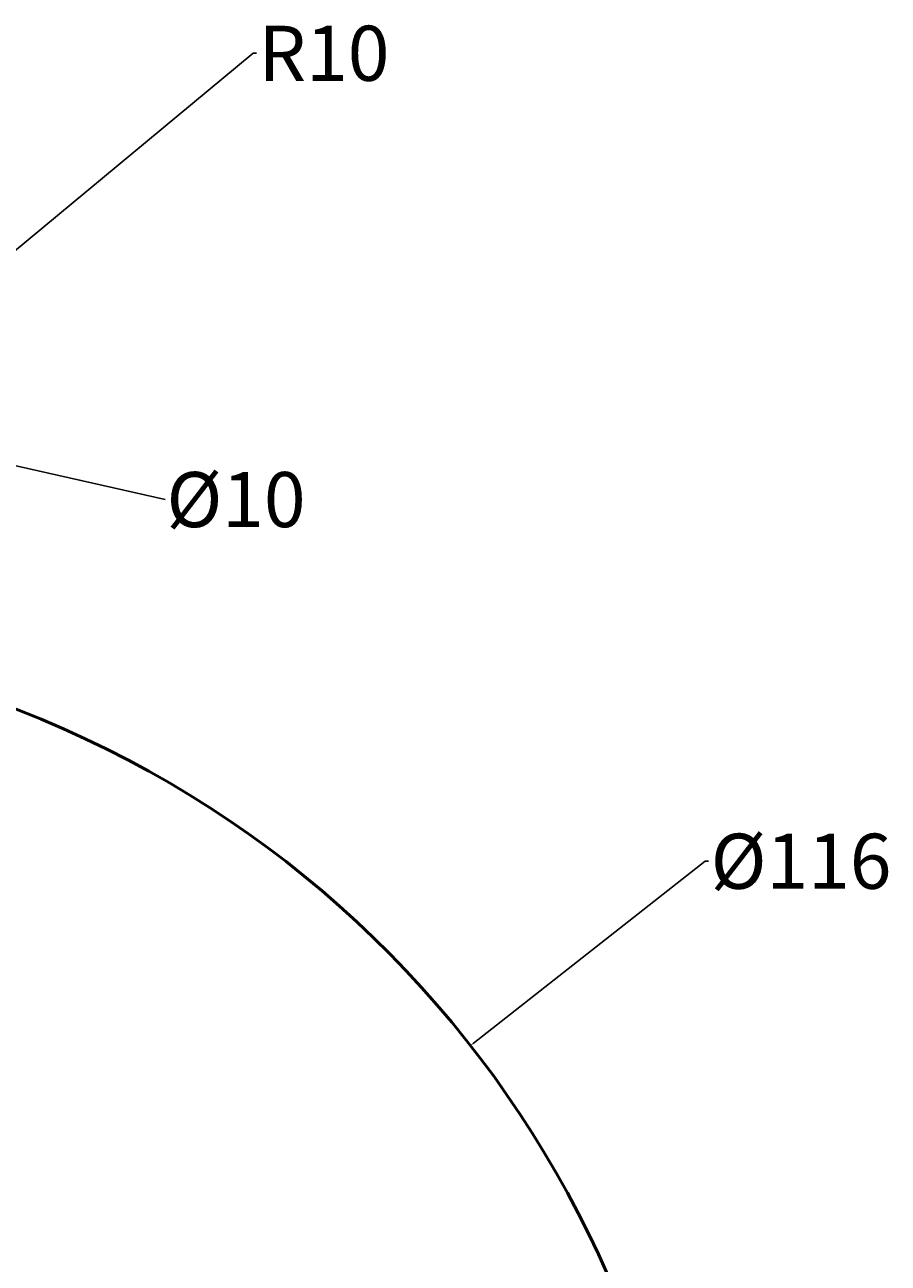
# Model space of a CAD drawing. Units: millimetres. Extents: x -53 to 92, y -147 to 37.
# Tile 16 of 16: x 40 to 87, y -30 to 37. Entities that reach past the tile are written whole.
import ezdxf

# ---------------------------------------------------------------- set-up
doc = ezdxf.new("R2010")
doc.units = ezdxf.units.MM
doc.header["$MEASUREMENT"] = 0
doc.layers.add('M-DIMS', color=2, linetype='Continuous', lineweight=25)
doc.layers.add('M-OUTL', color=7, linetype='Continuous', lineweight=50)
doc.styles.get("Standard").update_dxf_attribs({"font": 'arial.ttf'})
doc.dimstyles.get("Standard").update_dxf_attribs({"dimtxt": 0.18, "dimasz": 0.18, "dimexe": 0.18, "dimexo": 0.0625, "dimgap": 0.09, "dimtad": 0, "dimtih": 1, "dimtoh": 1, "dimdec": 4, "dimzin": 0, "dimdsep": 46, "dimtxsty": 'Standard', "dimcen": 0.09, "dimadec": 0, "dimazin": 0, "dimtfac": 1, "dimtdec": 4, "dimtofl": 0, "dimtmove": 0, "dimatfit": 3, "dimfxl": 1, "dimtolj": 1, "dimtzin": 0, "dimarcsym": 0})

# ---------------------------------------------------------------- blocks, each defined once
blk = doc.blocks.new('*D1')
at = {"layer": 'Defpoints', "color": 0, "transparency": 16777216}
for p in [(36.393, 22.289), (28.692, 15.91)]:
    blk.add_point(p, dxfattribs=at)
at = {"layer": 'M-DIMS', "color": 0, "lineweight": -2, "transparency": 16777216}
for p, q in [((52.762, 35.845), (36.532, 22.403)), ((52.942, 35.845), (52.762, 35.845)), ((28.602, 15.91), (28.782, 15.91)), ((28.692, 15.82), (28.692, 16))]:
    blk.add_line(p, q, dxfattribs=at)
at = {"layer": 'M-DIMS', "color": 0, "transparency": 16777216}
blk.add_solid([(36.513, 22.426), (36.551, 22.38), (36.393, 22.289)], dxfattribs=at)
at = {"layer": 'M-DIMS', "color": 0, "transparency": 16777216, "insert": (56.611, 35.845), "char_height": 0.18, "attachment_point": 5}
blk.add_mtext('\\A1;{\\H16.66667x;R10}', dxfattribs=at)
blk = doc.blocks.new('*D3')
at = {"layer": 'Defpoints', "color": 0, "transparency": 16777216}
for p in [(23.816, 17.015), (33.568, 14.805)]:
    blk.add_point(p, dxfattribs=at)
at = {"layer": 'M-DIMS', "color": 0, "lineweight": -2, "transparency": 16777216}
for p, q in [((28.602, 15.91), (28.782, 15.91)), ((28.692, 15.82), (28.692, 16)), ((47.959, 11.542), (33.744, 14.765))]:
    blk.add_line(p, q, dxfattribs=at)
at = {"layer": 'M-DIMS', "color": 0, "transparency": 16777216}
blk.add_solid([(33.75, 14.794), (33.737, 14.736), (33.568, 14.805)], dxfattribs=at)
at = {"layer": 'M-DIMS', "color": 0, "transparency": 16777216, "insert": (51.824, 11.542), "char_height": 0.18, "attachment_point": 5}
blk.add_mtext('\\A1;{\\H16.66667x;%%C10}', dxfattribs=at)
blk = doc.blocks.new('*D10')
at = {"layer": 'Defpoints', "color": 0, "transparency": 16777216}
for p in [(64.593, -18.184), (-26.68, -89.776)]:
    blk.add_point(p, dxfattribs=at)
at = {"layer": 'M-DIMS', "color": 0, "lineweight": -2, "transparency": 16777216}
for p, q in [((77.384, -8.151), (64.734, -18.073)), ((77.564, -8.151), (77.384, -8.151)), ((18.956, -54.07), (18.956, -53.89)), ((18.866, -53.98), (19.046, -53.98))]:
    blk.add_line(p, q, dxfattribs=at)
at = {"layer": 'M-DIMS', "color": 0, "transparency": 16777216}
blk.add_solid([(64.716, -18.05), (64.753, -18.097), (64.593, -18.184)], dxfattribs=at)
at = {"layer": 'M-DIMS', "color": 0, "transparency": 16777216, "insert": (82.599, -8.151), "char_height": 0.18, "attachment_point": 5}
blk.add_mtext('\\A1;{\\H16.66667x;%%C116}', dxfattribs=at)

msp = doc.modelspace()

# ---------------------------------------------------------------- linework, layer by layer
at = {"layer": 'M-OUTL'}
msp.add_arc((18.95638, -53.98007), 58, 108.3895553, 70.0459142, dxfattribs=at)

# ---------------------------------------------------------------- dimensions: what is measured, and where the dimension line sits
at = {"layer": 'M-DIMS'}
dim = msp.add_radius_dim(center=(28.69189, 15.91006), mpoint=(36.39347, 22.28858), text='{\\H16.66667x;R10}', dimstyle='Standard', override={"dimclrd": 0, "dimclre": 0, "dimclrt": 0}, dxfattribs=at)
dim.commit()
dim.dimension.update_dxf_attribs({"geometry": '*D1', "text_midpoint": (56.61093, 35.84496), "dimtype": 164})
for p1, p2, text, picture, middle in [((23.81561, 17.01547), (33.56816, 14.80464), '{\\H16.66667x;%%C10}', '*D3', (47.95869, 11.54241)), ((-26.67986, -89.77579), (64.59262, -18.18435), '{\\H16.66667x;%%C116}', '*D10', (82.59889, -8.15132))]:
    dim = msp.add_diameter_dim_2p(p1=p1, p2=p2, text=text, dimstyle='Standard', override={"dimclrd": 0, "dimclre": 0, "dimclrt": 0}, dxfattribs=at)
    dim.commit()
    dim.dimension.update_dxf_attribs({"geometry": picture, "text_midpoint": middle, "dimtype": 163})

doc.saveas('drawing.dxf')
